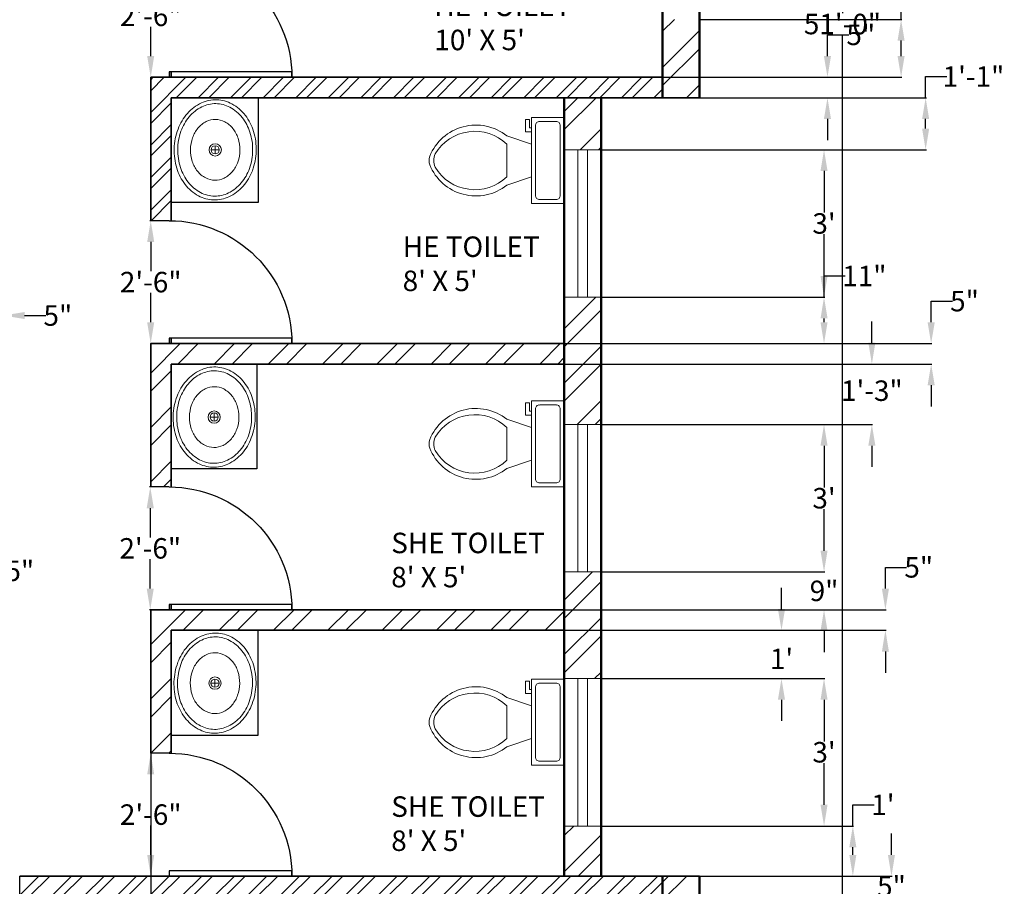
# Model space of a CAD drawing. Units: inches. Extents: x -355 to 263, y -871 to -163.
# Tile 4 of 6: x 23 to 263, y -733 to -521. Entities that reach past the tile are written whole.
import ezdxf

# ---------------------------------------------------------------- set-up
doc = ezdxf.new("R2010")
doc.units = ezdxf.units.IN
doc.header["$MEASUREMENT"] = 0
doc.layers.get('Defpoints').update_dxf_attribs({"color": 50})
for name, color, linetype, lineweight in [('A-ANNO-DIMS', 2, 'Continuous', 18), ('A-AREA-IDEN', 7, 'Continuous', 18), ('A-FLOR-CASE', 9, 'Continuous', 25), ('A-FLOR-FIXT', 8, 'Continuous', 18), ('A-WALL-PATT', 252, 'Continuous', 13)]:
    doc.layers.add(name, color=color, linetype=linetype, lineweight=lineweight)
for name, color, linetype, lineweight, plot in [('DOOR', 4, 'Continuous', 25, False), ('IWAL', 7, 'Continuous', 35, False), ('OWALL', 7, 'Continuous', 50, False), ('WIND', 3, 'Continuous', 18, False)]:
    doc.layers.add(name, color=color, linetype=linetype, lineweight=lineweight, plot=plot)
doc.styles.get("Standard").update_dxf_attribs({"font": 'arial.ttf'})
doc.dimstyles.get("Standard").update_dxf_attribs({"dimtxt": 5, "dimasz": 5.18, "dimexe": 0.18, "dimexo": 0.0625, "dimgap": 0.09, "dimtad": 0, "dimtih": 1, "dimtoh": 1, "dimdec": 0, "dimzin": 0, "dimdsep": 46, "dimlunit": 3, "dimtxsty": 'Standard', "dimcen": 0.09, "dimadec": 0, "dimazin": 0, "dimtfac": 1, "dimtdec": 0, "dimtofl": 0, "dimtmove": 0, "dimatfit": 3, "dimfxl": 1, "dimtolj": 1, "dimtzin": 0, "dimarcsym": 0})

# ---------------------------------------------------------------- blocks, each defined once
blk = doc.blocks.new('*U6')
for p, q in [((0, 0), (0, -6)), ((32, 0), (32, -6))]:
    blk.add_line(p, q)
blk.add_lwpolyline([(0, 0), (0, 32), (1.75, 32), (1.75, 0)], close=True)
blk.add_arc((0, 0), 32, 0, 90)
blk = doc.blocks.new('*U5')
for p, q in [((0, 0), (0, -6)), ((40, 0), (40, -6))]:
    blk.add_line(p, q)
blk.add_lwpolyline([(0, 0), (0, 40), (1.75, 40), (1.75, 0)], close=True)
blk.add_arc((0, 0), 40, 0, 90)
blk = doc.blocks.new('Toilet - top')
for p, q in [((9.5, -6), (9.5, -2)), ((-10, -8.5), (-8, -8.5)), ((-10, -9.5), (-10, -8.5)), ((-7, -9.5), (-10, -9.5)), ((-8, -8.5), (-8, -8)), ((-7, -8), (-7, -9.5)), ((-4, -8), (-6, -14)), ((4, -8), (6, -14)), ((4, -14), (-4, -14))]:
    blk.add_line(p, q)
blk.add_lwpolyline([(10.5, -8), (10.5, 0), (-10.5, 0), (-10.5, -8)], close=True)
for points in [[(-9.5, -2), (-9.5, -6)], [(8.5, -1), (-8.5, -1)], [(-8.5, -7), (8.5, -7)]]:
    blk.add_lwpolyline(points)
for centre, radius, start, end in [((-8.62, -1.88), 0.884, 81.8699, 188.1301), ((8.62, -1.88), 0.884, 351.8699, 98.1301), ((-8.62, -6.12), 0.884, 171.8699, 278.1301), ((8.62, -6.12), 0.884, 261.8699, 8.1301), ((3.52, -21.58), 12.17, 141.4691, 247.9714), ((4.2, -21.82), 11.33, 136.3677, 238.9468), ((-3.52, -21.58), 12.17, 292.0284, 38.5307), ((-4.2, -21.82), 11.33, 301.053, 43.6321), ((0, -27.88), 4, 245.7318, 294.2682), ((0, -29), 4, 254.8605, 285.1395)]:
    blk.add_arc(centre, radius, start, end)
blk = doc.blocks.new('Sink - Oval top')
for p, q in [((-1, 0), (1, 0)), ((0, 1), (0, -1))]:
    blk.add_line(p, q)
for points in [[(-12.23, 0.39, 0.117634), (-11.46, -3.36, 0.104469), (-8.88, -6.8, 0.090016), (-5.08, -9.07, 0.08192), (-0.32, -10.02, 0.08192), (4.49, -9.38, 0.090016), (8.42, -7.36, 0.104469), (11.22, -4.09, 0.117634), (12.23, -0.39, 0.117634), (11.46, 3.36, 0.104469), (8.88, 6.8, 0.090016), (5.08, 9.07, 0.08192), (0.32, 10.02, 0.08192), (-4.49, 9.38, 0.090016), (-8.42, 7.36, 0.104469), (-11.22, 4.09, 0.117634)], [(-11.29, 0.16, 0.118622), (-10.52, -3.25, 0.104678), (-8.07, -6.36, 0.089562), (-4.54, -8.37, 0.081185), (-0.13, -9.15, 0.081185), (4.3, -8.49, 0.089562), (7.89, -6.58, 0.104678), (10.42, -3.55, 0.118622), (11.29, -0.16, 0.118622), (10.52, 3.25, 0.104678), (8.07, 6.36, 0.089562), (4.54, 8.37, 0.081185), (0.13, 9.15, 0.081185), (-4.3, 8.49, 0.089562), (-7.89, 6.58, 0.104678), (-10.42, 3.55, 0.118622)], [(-7.42, 0.08, 0.118283), (-6.91, -2.17, 0.104607), (-5.29, -4.21, 0.089718), (-2.97, -5.53, 0.081436), (-0.07, -6.04, 0.081436), (2.84, -5.59, 0.089718), (5.2, -4.33, 0.104607), (6.86, -2.32, 0.118283), (7.42, -0.08, 0.118283), (6.91, 2.17, 0.104607), (5.29, 4.21, 0.089718), (2.97, 5.53, 0.081436), (0.07, 6.04, 0.081436), (-2.84, 5.59, 0.089718), (-5.2, 4.33, 0.104607), (-6.86, 2.32, 0.118283)]]:
    blk.add_lwpolyline(points, format="xyb", close=True)
for radius in [1.5, 1]:
    blk.add_circle((0, 0), radius)
blk = doc.blocks.new('*D14')
at = {"layer": 'A-ANNO-DIMS', "color": 0, "lineweight": -2, "transparency": 16777216}
for p, q in [((54.74, -700.29), (54.86, -700.29)), ((54.68, -705.47), (54.68, -712.64)), ((54.68, -725.1), (54.68, -717.93)), ((54.74, -730.28), (54.86, -730.28))]:
    blk.add_line(p, q, dxfattribs=at)
at = {"layer": 'A-ANNO-DIMS', "color": 0, "lineweight": -3, "transparency": 16777216}
for points in [[(53.82, -705.47), (55.54, -705.47), (54.68, -700.29)], [(53.82, -725.1), (55.54, -725.1), (54.68, -730.28)]]:
    blk.add_solid(points, dxfattribs=at)
at = {"layer": 'Defpoints', "color": 0, "lineweight": -3, "transparency": 16777216}
for p in [(54.68, -700.29), (54.68, -730.28), (54.68, -730.28)]:
    blk.add_point(p, dxfattribs=at)
at = {"layer": 'A-ANNO-DIMS', "color": 0, "transparency": 16777216, "insert": (54.68, -715.28), "char_height": 5, "attachment_point": 5}
blk.add_mtext('\\A1;2\'-6"', dxfattribs=at)
blk = doc.blocks.new('*D15')
at = {"layer": 'A-ANNO-DIMS', "color": 0, "lineweight": -2, "transparency": 16777216}
for p, q in [((54.62, -635.29), (54.39, -635.29)), ((54.57, -640.47), (54.57, -647.64)), ((54.57, -660.1), (54.57, -652.93)), ((54.62, -665.28), (54.39, -665.28))]:
    blk.add_line(p, q, dxfattribs=at)
at = {"layer": 'A-ANNO-DIMS', "color": 0, "lineweight": -3, "transparency": 16777216}
for points in [[(53.7, -640.47), (55.43, -640.47), (54.57, -635.29)], [(53.7, -660.1), (55.43, -660.1), (54.57, -665.28)]]:
    blk.add_solid(points, dxfattribs=at)
at = {"layer": 'Defpoints', "color": 0, "lineweight": -3, "transparency": 16777216}
for p in [(54.57, -635.29), (54.68, -635.29), (54.68, -665.28)]:
    blk.add_point(p, dxfattribs=at)
at = {"layer": 'A-ANNO-DIMS', "color": 0, "transparency": 16777216, "insert": (54.57, -650.28), "char_height": 5, "attachment_point": 5}
blk.add_mtext('\\A1;2\'-6"', dxfattribs=at)
blk = doc.blocks.new('*D16')
at = {"layer": 'A-ANNO-DIMS', "color": 0, "lineweight": -2, "transparency": 16777216}
for p, q in [((54.62, -570.29), (54.5, -570.29)), ((54.68, -575.47), (54.68, -582.64)), ((54.68, -595.1), (54.68, -587.93)), ((54.63, -600.28), (54.86, -600.28))]:
    blk.add_line(p, q, dxfattribs=at)
at = {"layer": 'A-ANNO-DIMS', "color": 0, "lineweight": -3, "transparency": 16777216}
for points in [[(53.82, -575.47), (55.54, -575.47), (54.68, -570.29)], [(53.82, -595.1), (55.54, -595.1), (54.68, -600.28)]]:
    blk.add_solid(points, dxfattribs=at)
at = {"layer": 'Defpoints', "color": 0, "lineweight": -3, "transparency": 16777216}
for p in [(54.68, -570.29), (54.68, -570.29), (54.57, -600.28)]:
    blk.add_point(p, dxfattribs=at)
at = {"layer": 'A-ANNO-DIMS', "color": 0, "transparency": 16777216, "insert": (54.68, -585.28), "char_height": 5, "attachment_point": 5}
blk.add_mtext('\\A1;2\'-6"', dxfattribs=at)
blk = doc.blocks.new('*D17')
at = {"layer": 'A-ANNO-DIMS', "color": 0, "lineweight": -2, "transparency": 16777216}
for p, q in [((54.62, -505.29), (54.5, -505.29)), ((54.68, -510.47), (54.68, -517.64)), ((54.68, -530.1), (54.68, -522.93)), ((54.74, -535.28), (54.86, -535.28))]:
    blk.add_line(p, q, dxfattribs=at)
at = {"layer": 'A-ANNO-DIMS', "color": 0, "lineweight": -3, "transparency": 16777216}
for points in [[(53.82, -510.47), (55.54, -510.47), (54.68, -505.29)], [(53.82, -530.1), (55.54, -530.1), (54.68, -535.28)]]:
    blk.add_solid(points, dxfattribs=at)
at = {"layer": 'Defpoints', "color": 0, "lineweight": -3, "transparency": 16777216}
for p in [(54.68, -505.29), (54.68, -505.29), (54.68, -535.28)]:
    blk.add_point(p, dxfattribs=at)
at = {"layer": 'A-ANNO-DIMS', "color": 0, "transparency": 16777216, "insert": (54.68, -520.28), "char_height": 5, "attachment_point": 5}
blk.add_mtext('\\A1;2\'-6"', dxfattribs=at)
blk = doc.blocks.new('*D18')
at = {"layer": 'A-ANNO-DIMS', "color": 0, "lineweight": -2, "transparency": 16777216}
for p, q in [((219.97, -530.1), (219.97, -524.92)), ((219.97, -524.92), (225.15, -524.92)), ((179.74, -535.28), (220.15, -535.28)), ((188.74, -540.28), (220.15, -540.28)), ((219.97, -545.46), (219.97, -550.64))]:
    blk.add_line(p, q, dxfattribs=at)
at = {"layer": 'A-ANNO-DIMS', "color": 0, "lineweight": -3, "transparency": 16777216}
for points in [[(219.1, -530.1), (220.83, -530.1), (219.97, -535.28)], [(219.1, -545.46), (220.83, -545.46), (219.97, -540.28)]]:
    blk.add_solid(points, dxfattribs=at)
at = {"layer": 'Defpoints', "color": 0, "lineweight": -3, "transparency": 16777216}
for p in [(179.68, -535.28), (219.97, -535.28), (188.68, -540.28)]:
    blk.add_point(p, dxfattribs=at)
at = {"layer": 'A-ANNO-DIMS', "color": 0, "transparency": 16777216, "insert": (228.11, -524.92), "char_height": 5, "attachment_point": 5}
blk.add_mtext('\\A1;5"', dxfattribs=at)
blk = doc.blocks.new('*D19')
at = {"layer": 'A-ANNO-DIMS', "color": 0, "lineweight": -2, "transparency": 16777216}
for p, q in [((237.95, -521.16), (237.95, -515.98)), ((237.95, -515.98), (243.13, -515.98)), ((188.74, -521.16), (238.13, -521.16)), ((237.95, -530.1), (237.95, -526.34)), ((179.74, -535.28), (238.13, -535.28))]:
    blk.add_line(p, q, dxfattribs=at)
at = {"layer": 'A-ANNO-DIMS', "color": 0, "lineweight": -3, "transparency": 16777216}
for points in [[(237.09, -526.34), (238.81, -526.34), (237.95, -521.16)], [(237.09, -530.1), (238.81, -530.1), (237.95, -535.28)]]:
    blk.add_solid(points, dxfattribs=at)
at = {"layer": 'Defpoints', "color": 0, "lineweight": -3, "transparency": 16777216}
for p in [(188.68, -521.16), (237.95, -521.16), (179.68, -535.28)]:
    blk.add_point(p, dxfattribs=at)
at = {"layer": 'A-ANNO-DIMS', "color": 0, "transparency": 16777216, "insert": (249.63, -515.98), "char_height": 5, "attachment_point": 5}
blk.add_mtext('\\A1;1\'-2"', dxfattribs=at)
blk = doc.blocks.new('*D29')
at = {"layer": 'A-ANNO-DIMS', "color": 0, "lineweight": -2, "transparency": 16777216}
for p, q in [((164.74, -682.06), (219.31, -682.06)), ((219.13, -687.24), (219.13, -697.41)), ((219.13, -712.88), (219.13, -702.7)), ((164.74, -718.06), (219.31, -718.06))]:
    blk.add_line(p, q, dxfattribs=at)
at = {"layer": 'A-ANNO-DIMS', "color": 0, "lineweight": -3, "transparency": 16777216}
for points in [[(218.27, -687.24), (219.99, -687.24), (219.13, -682.06)], [(218.27, -712.88), (219.99, -712.88), (219.13, -718.06)]]:
    blk.add_solid(points, dxfattribs=at)
at = {"layer": 'Defpoints', "color": 0, "lineweight": -3, "transparency": 16777216}
for p in [(164.68, -682.06), (219.13, -682.06), (164.68, -718.06)]:
    blk.add_point(p, dxfattribs=at)
at = {"layer": 'A-ANNO-DIMS', "color": 0, "transparency": 16777216, "insert": (219.13, -700.06), "char_height": 5, "attachment_point": 5}
blk.add_mtext("\\A1;3'", dxfattribs=at)
blk = doc.blocks.new('*D30')
at = {"layer": 'A-ANNO-DIMS', "color": 0, "lineweight": -2, "transparency": 16777216}
for p, q in [((208.74, -665.1), (208.74, -659.92)), ((155.74, -670.28), (208.92, -670.28)), ((164.74, -682.06), (208.92, -682.06)), ((208.74, -687.24), (208.74, -692.42))]:
    blk.add_line(p, q, dxfattribs=at)
at = {"layer": 'A-ANNO-DIMS', "color": 0, "lineweight": -3, "transparency": 16777216}
for points in [[(207.87, -665.1), (209.6, -665.1), (208.74, -670.28)], [(207.87, -687.24), (209.6, -687.24), (208.74, -682.06)]]:
    blk.add_solid(points, dxfattribs=at)
at = {"layer": 'Defpoints', "color": 0, "lineweight": -3, "transparency": 16777216}
for p in [(155.68, -670.28), (208.74, -670.28), (164.68, -682.06)]:
    blk.add_point(p, dxfattribs=at)
at = {"layer": 'A-ANNO-DIMS', "color": 0, "transparency": 16777216, "insert": (208.74, -677.26), "char_height": 5, "attachment_point": 5}
blk.add_mtext("\\A1;1'", dxfattribs=at)
blk = doc.blocks.new('*D31')
at = {"layer": 'A-ANNO-DIMS', "color": 0, "lineweight": -2, "transparency": 16777216}
for p, q in [((234.12, -660.1), (234.12, -654.92)), ((234.12, -654.92), (239.3, -654.92)), ((155.74, -665.28), (234.3, -665.28)), ((155.74, -670.28), (234.3, -670.28)), ((234.12, -675.46), (234.12, -680.64))]:
    blk.add_line(p, q, dxfattribs=at)
at = {"layer": 'A-ANNO-DIMS', "color": 0, "lineweight": -3, "transparency": 16777216}
for points in [[(233.26, -660.1), (234.98, -660.1), (234.12, -665.28)], [(233.26, -675.46), (234.98, -675.46), (234.12, -670.28)]]:
    blk.add_solid(points, dxfattribs=at)
at = {"layer": 'Defpoints', "color": 0, "lineweight": -3, "transparency": 16777216}
for p in [(155.68, -665.28), (234.12, -665.28), (155.68, -670.28)]:
    blk.add_point(p, dxfattribs=at)
at = {"layer": 'A-ANNO-DIMS', "color": 0, "transparency": 16777216, "insert": (242.26, -654.92), "char_height": 5, "attachment_point": 5}
blk.add_mtext('\\A1;5"', dxfattribs=at)
blk = doc.blocks.new('*D32')
at = {"layer": 'A-ANNO-DIMS', "color": 0, "lineweight": -2, "transparency": 16777216}
for p, q in [((219.13, -650.86), (219.13, -645.68)), ((164.74, -656.04), (219.31, -656.04)), ((155.74, -665.28), (219.31, -665.28)), ((219.13, -670.46), (219.13, -675.64))]:
    blk.add_line(p, q, dxfattribs=at)
at = {"layer": 'A-ANNO-DIMS', "color": 0, "lineweight": -3, "transparency": 16777216}
for points in [[(218.27, -650.86), (219.99, -650.86), (219.13, -656.04)], [(218.27, -670.46), (219.99, -670.46), (219.13, -665.28)]]:
    blk.add_solid(points, dxfattribs=at)
at = {"layer": 'Defpoints', "color": 0, "lineweight": -3, "transparency": 16777216}
for p in [(164.68, -656.04), (219.13, -656.04), (155.68, -665.28)]:
    blk.add_point(p, dxfattribs=at)
at = {"layer": 'A-ANNO-DIMS', "color": 0, "transparency": 16777216, "insert": (219.13, -660.66), "char_height": 5, "attachment_point": 5}
blk.add_mtext('\\A1;9"', dxfattribs=at)
blk = doc.blocks.new('*D33')
at = {"layer": 'A-ANNO-DIMS', "color": 0, "lineweight": -2, "transparency": 16777216}
for p, q in [((164.74, -620.04), (219.31, -620.04)), ((219.13, -625.22), (219.13, -635.4)), ((219.13, -650.86), (219.13, -640.69)), ((164.74, -656.04), (219.31, -656.04))]:
    blk.add_line(p, q, dxfattribs=at)
at = {"layer": 'A-ANNO-DIMS', "color": 0, "lineweight": -3, "transparency": 16777216}
for points in [[(218.27, -625.22), (219.99, -625.22), (219.13, -620.04)], [(218.27, -650.86), (219.99, -650.86), (219.13, -656.04)]]:
    blk.add_solid(points, dxfattribs=at)
at = {"layer": 'Defpoints', "color": 0, "lineweight": -3, "transparency": 16777216}
for p in [(164.68, -620.04), (219.13, -620.04), (164.68, -656.04)]:
    blk.add_point(p, dxfattribs=at)
at = {"layer": 'A-ANNO-DIMS', "color": 0, "transparency": 16777216, "insert": (219.13, -638.04), "char_height": 5, "attachment_point": 5}
blk.add_mtext("\\A1;3'", dxfattribs=at)
blk = doc.blocks.new('*D34')
at = {"layer": 'A-ANNO-DIMS', "color": 0, "lineweight": -2, "transparency": 16777216}
for p, q in [((230.81, -600.1), (230.81, -594.92)), ((155.74, -605.28), (230.99, -605.28)), ((164.74, -620.04), (230.99, -620.04)), ((230.81, -625.22), (230.81, -630.4))]:
    blk.add_line(p, q, dxfattribs=at)
at = {"layer": 'A-ANNO-DIMS', "color": 0, "lineweight": -3, "transparency": 16777216}
for points in [[(229.95, -600.1), (231.67, -600.1), (230.81, -605.28)], [(229.95, -625.22), (231.67, -625.22), (230.81, -620.04)]]:
    blk.add_solid(points, dxfattribs=at)
at = {"layer": 'Defpoints', "color": 0, "lineweight": -3, "transparency": 16777216}
for p in [(155.68, -605.28), (230.81, -605.28), (164.68, -620.04)]:
    blk.add_point(p, dxfattribs=at)
at = {"layer": 'A-ANNO-DIMS', "color": 0, "transparency": 16777216, "insert": (230.81, -611.79), "char_height": 5, "attachment_point": 5}
blk.add_mtext('\\A1;1\'-3"', dxfattribs=at)
blk = doc.blocks.new('*D35')
at = {"layer": 'A-ANNO-DIMS', "color": 0, "lineweight": -2, "transparency": 16777216}
for p, q in [((245.29, -595.1), (245.29, -589.92)), ((245.29, -589.92), (250.47, -589.92)), ((155.74, -600.28), (245.47, -600.28)), ((155.74, -605.28), (245.47, -605.28)), ((245.29, -610.46), (245.29, -615.64))]:
    blk.add_line(p, q, dxfattribs=at)
at = {"layer": 'A-ANNO-DIMS', "color": 0, "lineweight": -3, "transparency": 16777216}
for points in [[(244.43, -595.1), (246.16, -595.1), (245.29, -600.28)], [(244.43, -610.46), (246.16, -610.46), (245.29, -605.28)]]:
    blk.add_solid(points, dxfattribs=at)
at = {"layer": 'Defpoints', "color": 0, "lineweight": -3, "transparency": 16777216}
for p in [(155.68, -600.28), (245.29, -600.28), (155.68, -605.28)]:
    blk.add_point(p, dxfattribs=at)
at = {"layer": 'A-ANNO-DIMS', "color": 0, "transparency": 16777216, "insert": (253.44, -589.92), "char_height": 5, "attachment_point": 5}
blk.add_mtext('\\A1;5"', dxfattribs=at)
blk = doc.blocks.new('*D36')
at = {"layer": 'A-ANNO-DIMS', "color": 0, "lineweight": -2, "transparency": 16777216}
for p, q in [((219.13, -588.97), (219.13, -583.79)), ((219.13, -583.79), (224.31, -583.79)), ((164.74, -588.97), (219.31, -588.97)), ((219.13, -595.1), (219.13, -594.15)), ((155.74, -600.28), (219.31, -600.28))]:
    blk.add_line(p, q, dxfattribs=at)
at = {"layer": 'A-ANNO-DIMS', "color": 0, "lineweight": -3, "transparency": 16777216}
for points in [[(218.27, -594.15), (219.99, -594.15), (219.13, -588.97)], [(218.27, -595.1), (219.99, -595.1), (219.13, -600.28)]]:
    blk.add_solid(points, dxfattribs=at)
at = {"layer": 'Defpoints', "color": 0, "lineweight": -3, "transparency": 16777216}
for p in [(164.68, -588.97), (219.13, -588.97), (155.68, -600.28)]:
    blk.add_point(p, dxfattribs=at)
at = {"layer": 'A-ANNO-DIMS', "color": 0, "transparency": 16777216, "insert": (228.98, -583.79), "char_height": 5, "attachment_point": 5}
blk.add_mtext('\\A1;11"', dxfattribs=at)
blk = doc.blocks.new('*D37')
at = {"layer": 'A-ANNO-DIMS', "color": 0, "lineweight": -2, "transparency": 16777216}
for p, q in [((164.74, -552.97), (219.31, -552.97)), ((219.13, -558.15), (219.13, -568.32)), ((219.13, -583.79), (219.13, -573.61)), ((164.74, -588.97), (219.31, -588.97))]:
    blk.add_line(p, q, dxfattribs=at)
at = {"layer": 'A-ANNO-DIMS', "color": 0, "lineweight": -3, "transparency": 16777216}
for points in [[(218.27, -558.15), (219.99, -558.15), (219.13, -552.97)], [(218.27, -583.79), (219.99, -583.79), (219.13, -588.97)]]:
    blk.add_solid(points, dxfattribs=at)
at = {"layer": 'Defpoints', "color": 0, "lineweight": -3, "transparency": 16777216}
for p in [(164.68, -552.97), (219.13, -552.97), (164.68, -588.97)]:
    blk.add_point(p, dxfattribs=at)
at = {"layer": 'A-ANNO-DIMS', "color": 0, "transparency": 16777216, "insert": (219.13, -570.97), "char_height": 5, "attachment_point": 5}
blk.add_mtext("\\A1;3'", dxfattribs=at)
blk = doc.blocks.new('*D38')
at = {"layer": 'A-ANNO-DIMS', "color": 0, "lineweight": -2, "transparency": 16777216}
for p, q in [((243.94, -540.28), (243.94, -535.1)), ((243.94, -535.1), (249.12, -535.1)), ((188.74, -540.28), (244.12, -540.28)), ((243.94, -547.79), (243.94, -545.46)), ((164.74, -552.97), (244.12, -552.97))]:
    blk.add_line(p, q, dxfattribs=at)
at = {"layer": 'A-ANNO-DIMS', "color": 0, "lineweight": -3, "transparency": 16777216}
for points in [[(243.08, -545.46), (244.81, -545.46), (243.94, -540.28)], [(243.08, -547.79), (244.81, -547.79), (243.94, -552.97)]]:
    blk.add_solid(points, dxfattribs=at)
at = {"layer": 'Defpoints', "color": 0, "lineweight": -3, "transparency": 16777216}
for p in [(188.68, -540.28), (243.94, -540.28), (164.68, -552.97)]:
    blk.add_point(p, dxfattribs=at)
at = {"layer": 'A-ANNO-DIMS', "color": 0, "transparency": 16777216, "insert": (255.62, -535.1), "char_height": 5, "attachment_point": 5}
blk.add_mtext('\\A1;1\'-1"', dxfattribs=at)
blk = doc.blocks.new('*D41')
at = {"layer": 'A-ANNO-DIMS', "color": 0, "lineweight": -2, "transparency": 16777216}
for p, q in [((235.6, -725.1), (235.6, -719.92)), ((188.74, -730.28), (235.78, -730.28)), ((179.74, -735.28), (235.78, -735.28)), ((235.6, -740.46), (235.6, -745.64))]:
    blk.add_line(p, q, dxfattribs=at)
at = {"layer": 'A-ANNO-DIMS', "color": 0, "lineweight": -3, "transparency": 16777216}
for points in [[(234.73, -725.1), (236.46, -725.1), (235.6, -730.28)], [(234.73, -740.46), (236.46, -740.46), (235.6, -735.28)]]:
    blk.add_solid(points, dxfattribs=at)
at = {"layer": 'Defpoints', "color": 0, "lineweight": -3, "transparency": 16777216}
for p in [(188.68, -730.28), (235.6, -730.28), (179.68, -735.28)]:
    blk.add_point(p, dxfattribs=at)
at = {"layer": 'A-ANNO-DIMS', "color": 0, "transparency": 16777216, "insert": (235.6, -732.78), "char_height": 5, "attachment_point": 5}
blk.add_mtext('\\A1;5"', dxfattribs=at)
blk = doc.blocks.new('*D42')
at = {"layer": 'A-ANNO-DIMS', "color": 0, "lineweight": -2, "transparency": 16777216}
for p, q in [((226.17, -718.06), (226.17, -712.88)), ((226.17, -712.88), (231.35, -712.88)), ((164.74, -718.06), (226.35, -718.06)), ((226.17, -725.1), (226.17, -723.24)), ((188.74, -730.28), (226.35, -730.28))]:
    blk.add_line(p, q, dxfattribs=at)
at = {"layer": 'A-ANNO-DIMS', "color": 0, "lineweight": -3, "transparency": 16777216}
for points in [[(225.3, -723.24), (227.03, -723.24), (226.17, -718.06)], [(225.3, -725.1), (227.03, -725.1), (226.17, -730.28)]]:
    blk.add_solid(points, dxfattribs=at)
at = {"layer": 'Defpoints', "color": 0, "lineweight": -3, "transparency": 16777216}
for p in [(164.68, -718.06), (226.17, -718.06), (188.68, -730.28)]:
    blk.add_point(p, dxfattribs=at)
at = {"layer": 'A-ANNO-DIMS', "color": 0, "transparency": 16777216, "insert": (233.5, -712.88), "char_height": 5, "attachment_point": 5}
blk.add_mtext("\\A1;1'", dxfattribs=at)
blk = doc.blocks.new('*D55')
at = {"layer": 'A-ANNO-DIMS', "color": 0, "lineweight": -2, "transparency": 16777216}
for p, q in [((18.62, -641.28), (18.5, -641.28)), ((18.68, -646.46), (18.68, -653.14)), ((18.68, -665.1), (18.68, -658.42)), ((-7.26, -670.28), (18.86, -670.28))]:
    blk.add_line(p, q, dxfattribs=at)
at = {"layer": 'A-ANNO-DIMS', "color": 0, "lineweight": -3, "transparency": 16777216}
for points in [[(17.82, -646.46), (19.54, -646.46), (18.68, -641.28)], [(17.82, -665.1), (19.54, -665.1), (18.68, -670.28)]]:
    blk.add_solid(points, dxfattribs=at)
at = {"layer": 'Defpoints', "color": 0, "lineweight": -3, "transparency": 16777216}
for p in [(18.68, -641.28), (18.68, -641.28), (-7.32, -670.28)]:
    blk.add_point(p, dxfattribs=at)
at = {"layer": 'A-ANNO-DIMS', "color": 0, "transparency": 16777216, "insert": (18.68, -655.78), "char_height": 5, "attachment_point": 5}
blk.add_mtext('\\A1;2\'-5"', dxfattribs=at)
blk = doc.blocks.new('*D56')
at = {"layer": 'A-ANNO-DIMS', "color": 0, "lineweight": -2, "transparency": 16777216}
for p, q in [((8.5, -593.44), (3.32, -593.44)), ((13.68, -595.07), (13.68, -593.26)), ((18.68, -595.07), (18.68, -593.26)), ((23.86, -593.44), (29.04, -593.44))]:
    blk.add_line(p, q, dxfattribs=at)
at = {"layer": 'A-ANNO-DIMS', "color": 0, "lineweight": -3, "transparency": 16777216}
for points in [[(8.5, -592.58), (8.5, -594.3), (13.68, -593.44)], [(23.86, -592.58), (23.86, -594.3), (18.68, -593.44)]]:
    blk.add_solid(points, dxfattribs=at)
at = {"layer": 'Defpoints', "color": 0, "lineweight": -3, "transparency": 16777216}
for p in [(18.68, -593.44), (13.68, -595.13), (18.68, -595.13)]:
    blk.add_point(p, dxfattribs=at)
at = {"layer": 'A-ANNO-DIMS', "color": 0, "transparency": 16777216, "insert": (32, -593.44), "char_height": 5, "attachment_point": 5}
blk.add_mtext('\\A1;5"', dxfattribs=at)
blk = doc.blocks.new('WIN-36IN-9IN-WALL')
for p, q in [((4.5, 36), (0, 36)), ((3.3, 36), (3.3, 0)), ((4.5, 36), (9, 36)), ((5.7, 36), (5.7, 0)), ((4.5, 0), (0, 0)), ((4.5, 0), (9, 0))]:
    blk.add_line(p, q)
blk = doc.blocks.new('*D76')
at = {"layer": 'A-ANNO-DIMS', "color": 0, "lineweight": -2, "transparency": 16777216}
for p, q in [((188.74, -216.28), (223.81, -216.28)), ((223.63, -221.46), (223.63, -519.64)), ((223.63, -823.1), (223.63, -524.92)), ((188.74, -828.28), (223.81, -828.28))]:
    blk.add_line(p, q, dxfattribs=at)
at = {"layer": 'A-ANNO-DIMS', "color": 0, "lineweight": -3, "transparency": 16777216}
for points in [[(222.77, -221.46), (224.49, -221.46), (223.63, -216.28)], [(222.77, -823.1), (224.49, -823.1), (223.63, -828.28)]]:
    blk.add_solid(points, dxfattribs=at)
at = {"layer": 'Defpoints', "color": 0, "lineweight": -3, "transparency": 16777216}
for p in [(188.68, -216.28), (223.63, -216.28), (188.68, -828.28)]:
    blk.add_point(p, dxfattribs=at)
at = {"layer": 'A-ANNO-DIMS', "color": 0, "transparency": 16777216, "insert": (223.63, -522.28), "char_height": 5, "attachment_point": 5}
blk.add_mtext('\\A1;51\'-0"', dxfattribs=at)
blk = doc.blocks.new('*D86')
at = {"layer": 'A-ANNO-DIMS', "color": 0, "lineweight": -2, "transparency": 16777216}
for p, q in [((18.68, -641.34), (18.68, -863.41)), ((54.68, -665.34), (54.68, -863.41)), ((23.86, -863.23), (29.95, -863.23)), ((49.5, -863.23), (43.41, -863.23))]:
    blk.add_line(p, q, dxfattribs=at)
at = {"layer": 'A-ANNO-DIMS', "color": 0, "lineweight": -3, "transparency": 16777216}
for points in [[(23.86, -862.37), (23.86, -864.09), (18.68, -863.23)], [(49.5, -862.37), (49.5, -864.09), (54.68, -863.23)]]:
    blk.add_solid(points, dxfattribs=at)
at = {"layer": 'Defpoints', "color": 0, "lineweight": -3, "transparency": 16777216}
for p in [(18.68, -641.28), (54.68, -665.28), (54.68, -863.23)]:
    blk.add_point(p, dxfattribs=at)
at = {"layer": 'A-ANNO-DIMS', "color": 0, "transparency": 16777216, "insert": (36.68, -863.23), "char_height": 5, "attachment_point": 5}
blk.add_mtext('\\A1;3\'-0"', dxfattribs=at)

msp = doc.modelspace()

# ---------------------------------------------------------------- hatches: boundary and pattern name
at = {"layer": 'A-WALL-PATT'}
h = msp.add_hatch(dxfattribs=at)
h.set_pattern_fill('ANSI32', color=256, scale=25)
h.set_pattern_definition([(45, (-301.32, -828.28), (-6.62913, 6.62913), []), (45, (-296.9, -828.28), (-6.62913, 6.62913), [])])
h.paths.add_polyline_path([(54.68, -289.28), (-301.32, -289.28), (-301.32, -303.28), (-295.02, -303.28), (-292.32, -303.28), (-292.32, -298.28), (54.68, -298.28)])
h.paths.add_polyline_path([(188.68, -216.28), (54.68, -216.28), (54.68, -225.28), (179.68, -225.28), (179.68, -345.28), (179.68, -485.16), (184.18, -485.16), (188.68, -485.16)])
h.paths.add_polyline_path([(188.68, -521.16), (184.18, -521.16), (179.68, -521.16), (179.68, -540.28), (188.68, -540.28)])
h.paths.add_polyline_path([(164.68, -540.28), (155.68, -540.28), (155.68, -552.97), (160.18, -552.97), (164.68, -552.97)])
h.paths.add_polyline_path([(164.68, -588.97), (160.18, -588.97), (155.68, -588.97), (155.68, -620.04), (160.18, -620.04), (164.68, -620.04)])
h.paths.add_polyline_path([(164.68, -656.04), (160.18, -656.04), (155.68, -656.04), (155.68, -682.06), (160.18, -682.06), (164.68, -682.06)])
h.paths.add_polyline_path([(164.68, -718.06), (160.18, -718.06), (155.68, -718.06), (155.68, -730.28), (164.68, -730.28)])
h.paths.add_polyline_path([(188.68, -730.28), (179.68, -730.28), (179.68, -819.28), (73.9, -819.28), (73.9, -823.78), (73.9, -828.28), (188.68, -828.28)])
h.paths.add_polyline_path([(25.9, -819.28), (-41.45, -819.28), (-41.45, -823.78), (-41.45, -828.28), (25.9, -828.28), (25.9, -823.78)])
h.paths.add_polyline_path([(-113.45, -819.28), (-292.32, -819.28), (-292.32, -796.14), (-296.82, -796.14), (-301.32, -796.14), (-301.32, -828.28), (-113.45, -828.28), (-113.45, -823.78)])
h.paths.add_polyline_path([(-292.32, -480.28), (-292.32, -345.28), (-301.32, -345.28), (-301.32, -620.18), (-296.82, -620.18), (-292.32, -620.18)])
h.paths.add_polyline_path([(-292.32, -656.18), (-296.82, -656.18), (-301.32, -656.18), (-301.32, -700.14), (-296.82, -700.14), (-292.32, -700.14)])
h = msp.add_hatch(dxfattribs=at)
h.set_pattern_fill('ANSI32', color=256, scale=15)
h.set_pattern_definition([(45, (-292.3197, -819.28), (-3.977476, 3.977476), []), (45, (-289.668, -819.28), (-3.977476, 3.977476), [])])
h.paths.add_polyline_path([(59.68, -280.18), (57.18, -280.18), (54.68, -280.18), (54.68, -289.28), (54.68, -298.28), (54.68, -303.28), (59.68, -303.28)])
h.paths.add_polyline_path([(59.68, -225.28), (54.68, -225.28), (54.68, -232.18), (57.18, -232.18), (59.68, -232.18)])
h.paths.add_polyline_path([(18.68, -641.28), (18.68, -521.28), (13.68, -521.28), (13.68, -641.28), (-7.32, -665.28), (-105.32, -665.28), (-126.32, -641.28), (-126.32, -521.28), (-131.32, -521.28), (-131.32, -641.28), (-105.32, -670.28), (-7.32, -670.28)])
h.paths.add_polyline_path([(-167.32, -521.28), (-172.32, -521.28), (-172.32, -538.25), (-169.82, -538.25), (-167.32, -538.25)])
h.paths.add_polyline_path([(-134.32, -670.28), (-167.32, -670.28), (-167.32, -610.28), (-167.32, -586.25), (-169.82, -586.25), (-172.32, -586.25), (-172.32, -670.28), (-292.32, -670.28), (-292.32, -675.28), (-139.32, -675.28), (-134.32, -675.28)])
h.paths.add_polyline_path([(-167.32, -345.28), (-172.32, -345.28), (-172.32, -462.28), (-172.32, -480.28), (-292.32, -480.28), (-292.32, -485.28), (-172.32, -485.28), (-167.32, -485.28), (5.68, -485.28), (5.68, -480.28), (-167.32, -480.28)])
h.paths.add_polyline_path([(179.68, -345.28), (30.68, -345.28), (30.68, -365.65), (33.18, -365.65), (35.68, -365.65), (35.68, -350.28), (179.68, -350.28)])
h.paths.add_polyline_path([(-134.32, -707.28), (-139.32, -707.28), (-139.32, -819.28), (-134.32, -819.28)])
h.paths.add_polyline_path([(-9.32, -707.28), (-102.32, -707.28), (-102.32, -712.28), (-14.32, -712.28), (-14.32, -819.28), (-9.32, -819.28)])
h.paths.add_polyline_path([(179.68, -730.28), (22.68, -730.28), (22.68, -735.28), (179.68, -735.28)])
h.paths.add_polyline_path([(179.68, -470.28), (30.68, -470.28), (30.68, -475.28), (54.68, -475.28), (54.68, -505.29), (59.18, -505.29, -0.00418), (59.68, -505.29), (59.68, -475.28), (179.68, -475.28)])
h.paths.add_polyline_path([(35.68, -413.65), (33.18, -413.65), (30.68, -413.65), (30.68, -440.29), (35.18, -440.29, -0.00418), (35.68, -440.29)])
h.paths.add_polyline_path([(179.68, -535.28), (54.68, -535.28), (54.68, -540.28), (54.68, -570.29), (59.18, -570.29, -0.00418), (59.68, -570.29), (59.68, -540.28), (179.68, -540.28)])
h.paths.add_polyline_path([(121.93, -531.51), (160.73, -531.51), (160.73, -512.85), (121.93, -512.85)], flags=9)
h.paths.add_polyline_path([(49.47, -376.48), (111.2, -376.48), (111.2, -357.82), (49.47, -357.82)], flags=9)
h = msp.add_hatch(dxfattribs=at)
h.set_pattern_fill('ANSI32', color=256, scale=25)
h.set_pattern_definition([(45, (54.68, -700.294), (-6.6291, 6.6291), []), (45, (59.1, -700.294), (-6.6291, 6.6291), [])])
h.paths.add_polyline_path([(155.68, -600.28), (54.68, -600.28), (54.68, -635.29), (59.18, -635.29, -0.00418), (59.68, -635.29), (59.68, -605.28), (155.68, -605.28)])
h.paths.add_polyline_path([(155.68, -665.28), (54.68, -665.28), (54.68, -700.29), (59.18, -700.29, -0.00418), (59.68, -700.29), (59.68, -670.28), (155.68, -670.28)])

# ---------------------------------------------------------------- linework, layer by layer
at = {"layer": 'A-FLOR-CASE'}
for p, q in [((80.9, -540.28), (80.9, -540.28)), ((80.9, -540.28), (80.9, -565.82)), ((80.9, -565.82), (59.68, -565.82)), ((80.56, -605.28), (80.56, -630.84)), ((80.56, -630.84), (59.68, -630.84)), ((80.84, -670.28), (80.84, -695.96)), ((80.84, -695.96), (59.68, -695.96))]:
    msp.add_line(p, q, dxfattribs=at)
at = {"layer": 'IWAL'}
for p, q in [((179.68, -535.28), (54.68, -535.28)), ((54.68, -535.28), (54.68, -570.29)), ((54.68, -535.28), (54.68, -540.28)), ((59.68, -533.97), (59.68, -535.28)), ((188.68, -540.28), (59.68, -540.28)), ((59.68, -540.28), (59.68, -570.29)), ((155.68, -600.28), (54.68, -600.28)), ((54.68, -600.28), (54.68, -635.29)), ((59.68, -598.97), (59.68, -600.28)), ((155.68, -605.28), (59.68, -605.28)), ((59.68, -605.28), (59.68, -635.29)), ((155.68, -665.28), (54.68, -665.28)), ((54.68, -665.28), (54.68, -700.29)), ((59.68, -663.97), (59.68, -665.28)), ((59.68, -670.28), (59.68, -700.29)), ((155.68, -670.28), (59.68, -670.28)), ((188.68, -730.28), (22.68, -730.28))]:
    msp.add_line(p, q, dxfattribs=at)
at = {"layer": 'OWALL'}
for p, q in [((188.68, -216.28), (188.68, -540.28)), ((179.68, -345.28), (179.68, -540.28)), ((155.68, -540.28), (155.68, -730.28)), ((164.68, -540.28), (164.68, -730.28)), ((179.68, -730.28), (179.68, -819.28)), ((188.68, -730.28), (188.68, -828.28))]:
    msp.add_line(p, q, dxfattribs=at)

# ---------------------------------------------------------------- block references
at = {"layer": 'A-FLOR-FIXT'}
for name, p, rotation in [('Sink - Oval top', (70.43, -553), 90), ('Toilet - top', (155.68, -555.6), 269.9999999999998), ('Sink - Oval top', (70.18, -618.23), 90), ('Toilet - top', (155.68, -624.78), 269.9999999999998), ('Sink - Oval top', (70.38, -683.18), 90), ('Toilet - top', (155.68, -692.72), 269.9999999999998)]:
    msp.add_blockref(name, p, dxfattribs=dict(at, rotation=rotation))
at = {"layer": 'DOOR', "xscale": -0.7497657348060921, "yscale": 0.7497657348060921, "zscale": 0.7497657348060921, "rotation": 270}
for p in [(59.18, -535.28), (59.18, -600.28), (59.18, -665.28), (59.18, -730.28)]:
    msp.add_blockref('*U5', p, dxfattribs=at)
at = {"layer": 'DOOR', "xscale": -1, "rotation": 180}
msp.add_blockref('*U6', (-9.32, -736.28), dxfattribs=at)
at = {"layer": 'WIND'}
for p in [(155.68, -588.97), (155.68, -656.04), (155.68, -718.06)]:
    msp.add_blockref('WIN-36IN-9IN-WALL', p, dxfattribs=at)

# ---------------------------------------------------------------- texts
at = {"layer": 'A-AREA-IDEN', "char_height": 5, "attachment_point": 1}
for s, width, insert in [("{HE TOILET\\P10' X 5'}", 50.5823, (123.95, -515.34)), ("{HE TOILET\\P8' X 5'}", 38.3562, (116.22, -574.14)), ("{SHE TOILET\\P8' X 5'}", 101.484, (113.42, -646.46)), ("{SHE TOILET\\P8' X 5'}", 101.484, (113.42, -710.82))]:
    msp.add_mtext_dynamic_manual_height_columns(s, width=width, gutter_width=1, heights=[0], dxfattribs=dict(at, insert=insert))

# ---------------------------------------------------------------- dimensions: what is measured, and where the dimension line sits
at = {"layer": 'A-ANNO-DIMS'}
for base, p1, p2, angle, override, picture, middle in [((223.63, -216.28), (188.68, -828.28), (188.68, -216.28), 90, {"dimdec": 1, "dimlfac": 1, "dimrnd": 0, "dimzin": 1, "dimdsep": 46, "dimlunit": 4, "dimfrac": 2}, '*D76', (223.63, -522.28)), ((54.68, -505.29), (54.68, -535.28), (54.68, -505.29), 90, {"dimclrd": 0, "dimclre": 0, "dimclrt": 0}, '*D17', (54.68, -520.28)), ((237.95, -521.16), (179.68, -535.28), (188.68, -521.16), 270, {"dimclrd": 0, "dimclre": 0, "dimclrt": 0}, '*D19', (249.63, -515.98)), ((219.97, -535.28), (188.68, -540.28), (179.68, -535.28), 270, {"dimclrd": 0, "dimclre": 0, "dimclrt": 0}, '*D18', (228.11, -524.92)), ((243.94, -540.28), (164.68, -552.97), (188.68, -540.28), 270, {"dimclrd": 0, "dimclre": 0, "dimclrt": 0}, '*D38', (255.62, -535.1)), ((219.13, -552.97), (164.68, -588.97), (164.68, -552.97), 270, {"dimclrd": 0, "dimclre": 0, "dimclrt": 0}, '*D37', (219.13, -570.97)), ((54.68, -570.29), (54.57, -600.28), (54.68, -570.29), 90, {"dimclrd": 0, "dimclre": 0, "dimclrt": 0}, '*D16', (54.68, -585.28)), ((219.13, -588.97), (155.68, -600.28), (164.68, -588.97), 270, {"dimclrd": 0, "dimclre": 0, "dimclrt": 0}, '*D36', (228.98, -583.79)), ((219.13, -620.04), (164.68, -656.04), (164.68, -620.04), 270, {"dimclrd": 0, "dimclre": 0, "dimclrt": 0}, '*D33', (219.13, -638.04)), ((54.57, -635.29), (54.68, -665.28), (54.68, -635.29), 90, {"dimclrd": 0, "dimclre": 0, "dimclrt": 0}, '*D15', (54.57, -650.28)), ((18.68, -641.28), (-7.32, -670.28), (18.68, -641.28), 90, {"dimclrd": 0, "dimclre": 0, "dimclrt": 0}, '*D55', (18.68, -655.78)), ((219.13, -656.04), (155.68, -665.28), (164.68, -656.04), 270, {"dimclrd": 0, "dimclre": 0, "dimclrt": 0}, '*D32', (219.13, -660.66)), ((234.12, -665.28), (155.68, -670.28), (155.68, -665.28), 270, {"dimclrd": 0, "dimclre": 0, "dimclrt": 0}, '*D31', (242.26, -654.92)), ((219.13, -682.06), (164.68, -718.06), (164.68, -682.06), 270, {"dimclrd": 0, "dimclre": 0, "dimclrt": 0}, '*D29', (219.13, -700.06)), ((54.68, -730.28), (54.68, -700.29), (54.68, -730.28), 90, {"dimclrd": 0, "dimclre": 0, "dimclrt": 0}, '*D14', (54.68, -715.28))]:
    dim = msp.add_linear_dim(base=base, p1=p1, p2=p2, angle=angle, dimstyle='Standard', override=override, dxfattribs=at)
    dim.commit()
    dim.dimension.update_dxf_attribs({"geometry": picture, "text_midpoint": middle})
for base, p1, p2, picture, middle in [((245.29, -600.28), (155.68, -605.28), (155.68, -600.28), '*D35', (253.44, -589.92)), ((230.81, -605.28), (164.68, -620.04), (155.68, -605.28), '*D34', (230.81, -611.79)), ((208.74, -670.28), (164.68, -682.06), (155.68, -670.28), '*D30', (208.74, -677.26)), ((226.17, -718.06), (188.68, -730.28), (164.68, -718.06), '*D42', (233.5, -712.88)), ((235.6, -730.28), (179.68, -735.28), (188.68, -730.28), '*D41', (235.6, -732.78))]:
    dim = msp.add_linear_dim(base=base, p1=p1, p2=p2, angle=270, dimstyle='Standard', override={"dimclrd": 0, "dimclre": 0, "dimclrt": 0}, dxfattribs=at)
    dim.commit()
    dim.dimension.update_dxf_attribs({"geometry": picture, "text_midpoint": middle, "dimtype": 160})
for base, p1, p2, override, picture, middle in [((18.68, -593.44), (13.68, -595.13), (18.68, -595.13), {"dimclrd": 0, "dimclre": 0, "dimclrt": 0}, '*D56', (32, -593.44)), ((54.68, -863.23), (18.68, -641.28), (54.68, -665.28), {"dimdec": 1, "dimlfac": 1, "dimrnd": 0, "dimzin": 1, "dimdsep": 46, "dimlunit": 4, "dimfrac": 2}, '*D86', (36.68, -863.23))]:
    dim = msp.add_linear_dim(base=base, p1=p1, p2=p2, dimstyle='Standard', override=override, dxfattribs=at)
    dim.commit()
    dim.dimension.update_dxf_attribs({"geometry": picture, "text_midpoint": middle})

doc.saveas('drawing.dxf')
